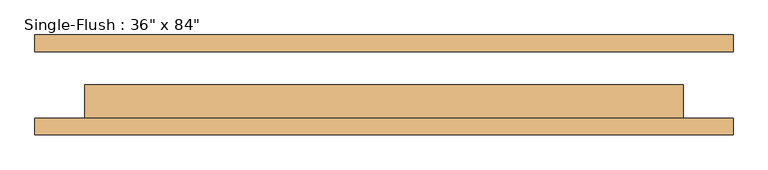
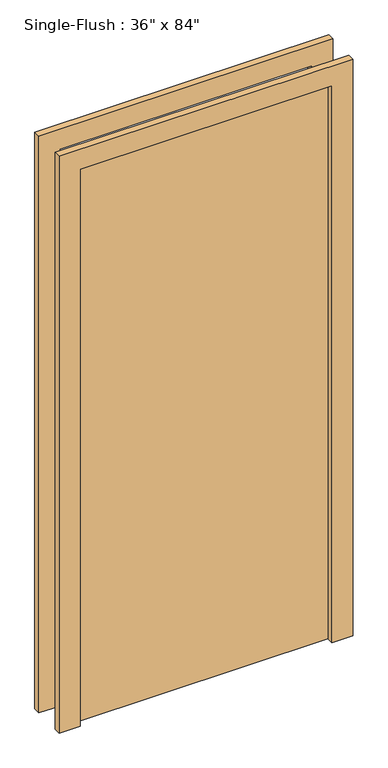
"""IFC4 building model written with IfcOpenShell, lengths in millimetres: door geometry."""

from ifc_helpers import new_model, si_unit, frame, origin, origin_with_axes, place, context, project, spatial, polyline, outline, extrude, source, transform, mapped, element, save


def door_310a3c6c(model_context):
    return source(origin(), model_context, "Body", "SweptSolid", [
        extrude(outline(polyline([(2209.8, -533.4), (0.0, -533.4), (0.0, -457.2), (2133.6, -457.2), (2133.6, 457.2), (0.0, 457.2), (0.0, 533.4), (2209.8, 533.4), (2209.8, -533.4)])), frame((0.0, -76.2, 0.0), z_axis=(0.0, 1.0, 0.0), x_axis=(0.0, 0.0, 1.0)), (0.0, 0.0, 1.0), 25.4),
        extrude(outline(polyline([(2209.8, 533.4), (2209.8, -533.4), (0.0, -533.4), (0.0, -457.2), (2133.6, -457.2), (2133.6, 457.2), (0.0, 457.2), (0.0, 533.4), (2209.8, 533.4)])), frame((0.0, 50.8, 0.0), z_axis=(0.0, 1.0, 0.0), x_axis=(0.0, 0.0, 1.0)), (0.0, 0.0, 1.0), 25.4),
        extrude(outline(polyline([(457.2, 0.0), (457.2, -50.8), (-457.2, -50.8), (-457.2, 0.0), (457.2, 0.0)])), origin_with_axes(), (0.0, 0.0, 1.0), 2133.6),
    ])


if __name__ == "__main__":
    model = new_model("IFC4")
    model_context = context("Model", 3, world=origin())
    ifc_project = project(units=[si_unit("LENGTHUNIT", "METRE", prefix="MILLI")], contexts=[model_context])
    site = spatial("IfcSite", under=ifc_project)
    building = spatial("IfcBuilding", under=site)
    placement = place(None, origin())
    door_shape = door_310a3c6c(model_context)
    element("IfcDoor", 1, ObjectType="Single-Flush : 36\" x 84\"", at=placement, inside=building, context=model_context, shape_type="MappedRepresentation", body=[
        mapped(door_shape, transform((0.0, 0.0, 0.0), x_axis=(1.0, 0.0, 0.0), y_axis=(0.0, 1.0, 0.0), z_axis=(0.0, 0.0, 1.0))),
    ])
    save(model, "model.ifc")

# Revit data of these elements
# Type "Single-Flush : 36\" x 84\""
#   Type Mark = "5"
#   Construction Type Id = "MDOOR"
#   Assembly Code = "C1020"
#   Analytic Construction = "Metal"
#   Thickness = 0' - 2"
#   Heat Transfer Coefficient (U) = 0.651978 BTU/(h·ft²·°F)
#   Height = 7' - 0"
#   Trim Projection Ext = 0' - 1"
#   Trim Projection Int = 0' - 1"
#   Trim Width = 0' - 3"
#   Width = 3' - 0"
#   Define Thermal Properties by = 1
#   Define Thermal Properties by = 1
#   Door Material = Door - Panel
#   Frame Material = Door - Frame
#   Visual Light Transmittance = 0
#   Solar Heat Gain Coefficient = 0
#   Function = (empty or 0)
#   Wall Closure = (empty or 0)
# Element 1 (IfcDoor, "Single-Flush : 36\" x 84\"")
#   Materials on its faces: "Door - Frame", "Door - Panel"
# Materials
#   "Door - Panel": class "Wood", colour RGB 210 159 95, transparency 0, Cost = 0
#   "Door - Frame": colour RGB 118 70 51, transparency 0, Cost = 0
